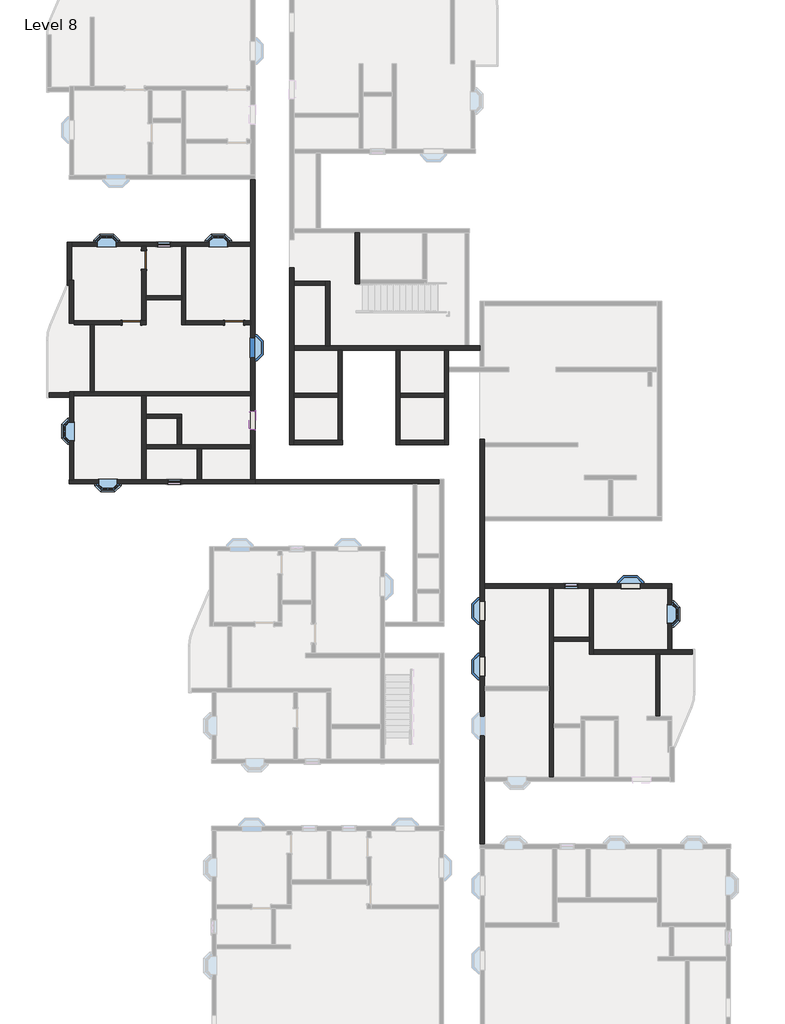
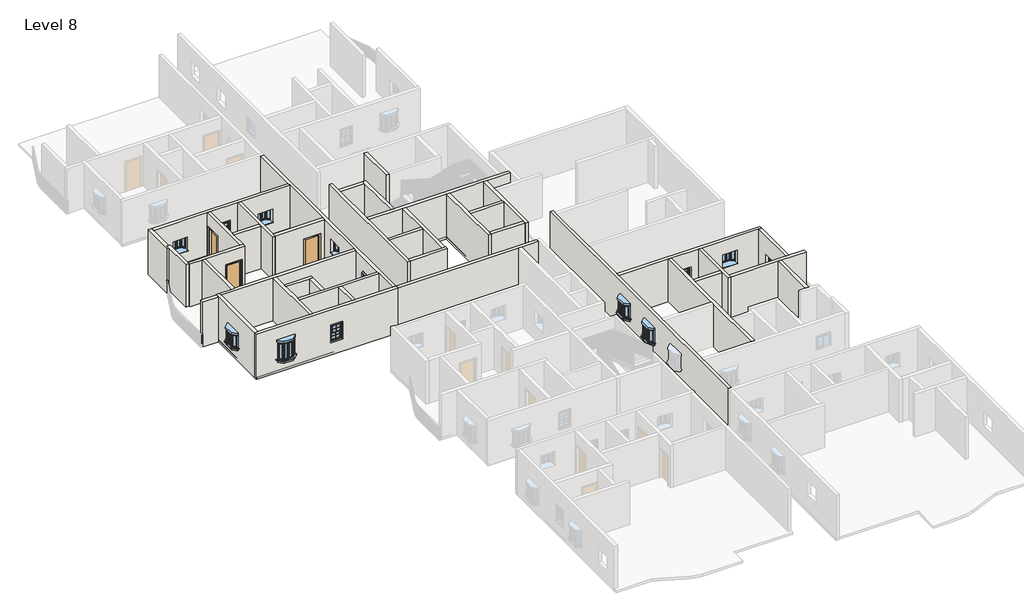
# One storey, part 3 of 14: 40 walls, 13 windows, 3 doors.
# Revit data of these elements (continued)
# Element 25 (IfcWall, "9\"")
#   Top Offset = 0' - 0"
#   Base Offset = 0' - 0"
#   wall height = 10' - 0"
#   Phase Created = New Construction
#   Base Constraint = Level 8
#   Top Constraint = Level 9
#   Materials on its faces: "Default Wall", "Parking Stripe"
# Element 26 (IfcWall, "9\"")
#   Top Offset = 0' - 0"
#   Base Offset = 0' - 0"
#   wall height = 10' - 0"
#   Phase Created = New Construction
#   Base Constraint = Level 8
#   Top Constraint = Level 9
#   Materials on its faces: "Default Wall", "Earth"
# Element 27 (IfcWall, "9\"")
#   Top Offset = 0' - 0"
#   Base Offset = 0' - 0"
#   wall height = 10' - 0"
#   Phase Created = New Construction
#   Base Constraint = Level 8
#   Top Constraint = Level 9
#   Materials on its faces: "Default Wall", "Default Mass Interior Wall"
# Element 28 (IfcWall, "9\"")
#   Top Offset = 0' - 0"
#   Base Offset = 0' - 0"
#   wall height = 10' - 0"
#   Phase Created = New Construction
#   Base Constraint = Level 8
#   Top Constraint = Level 9
#   Materials on its faces: "Default Wall"
# Element 29 (IfcWall, "9\"")
#   Top Offset = 0' - 0"
#   Base Offset = 0' - 0"
#   wall height = 10' - 0"
#   Phase Created = New Construction
#   Base Constraint = Level 8
#   Top Constraint = Level 9
#   Materials on its faces: "Default Wall", "Default Mass Interior Wall", "Earth"
# Elements 30, 33, 34, 35, 36, 37, 38, 39, 40, 41 (IfcWall, "9\" w")
#   Top Offset = 0' - 0"
#   Base Offset = 0' - 0"
#   wall height = 10' - 0"
#   Phase Created = New Construction
#   Base Constraint = Level 8
#   Top Constraint = Level 9
#   Materials on its faces: "Default Wall"
# Element 31 (IfcWall, "9\" w")
#   Top Offset = 0' - 0"
#   Base Offset = 0' - 0"
#   wall height = 10' - 0"
#   Phase Created = New Construction
#   Base Constraint = Level 8
#   Top Constraint = Level 9
#   Materials on its faces: "Default Wall", "Earth"
# Element 32 (IfcWall, "9\" w")
#   Top Offset = 0' - 0"
#   Base Offset = 0' - 0"
#   wall height = 10' - 0"
#   Phase Created = New Construction
#   Base Constraint = Level 8
#   Top Constraint = Level 9
#   Materials on its faces: "Default Wall", "Brick, Soldier Course"
# Element 42 (IfcWall, "9\" w")
#   Top Offset = 0' - 0"
#   Base Offset = 0' - 0"
#   wall height = 10' - 0"
#   Phase Created = New Construction
#   Base Constraint = Level 8
#   Top Constraint = Level 9
#   Materials on its faces: "Default Wall", "Wood - Stained"
# Element 43 (IfcWall, "9\" w")
#   Top Offset = 0' - 0"
#   Base Offset = 0' - 0"
#   wall height = 10' - 0"
#   Phase Created = New Construction
#   Base Constraint = Level 8
#   Top Constraint = Level 9
#   Materials on its faces: "Default Wall", "Acoustic Ceiling Tile 24 x 24"
# Element 44 (IfcWindow, "910x1210mm")
#   Mark = "471"
#   Phase Created = New Construction
#   Materials on its faces: "Window Frame", "Glass"
# Element 45 (IfcWindow, "910x910mm")
#   Mark = "447"
#   Phase Created = New Construction
#   Materials on its faces: "Window Frame", "Glass"
# Element 46 (IfcWindow, "910x910mm")
#   Mark = "448"
#   Phase Created = New Construction
#   Materials on its faces: "Window Frame", "Glass"
# Element 47 (IfcWindow, "910x910mm")
#   Mark = "420"
#   Phase Created = New Construction
#   Materials on its faces: "Window Frame", "Glass"
# Element 48 (IfcWindow, "910x910mm")
#   Mark = "421"
#   Phase Created = New Construction
#   Materials on its faces: "Window Frame", "Glass"
# Element 49 (IfcWindow, "910x910mm")
#   Mark = "422"
#   Phase Created = New Construction
#   Materials on its faces: "Window Frame", "Glass"
# Element 50 (IfcWindow, "910x910mm")
#   Mark = "423"
#   Phase Created = New Construction
#   Materials on its faces: "Window Frame", "Glass"
# Element 51 (IfcWindow, "910x910mm")
#   Mark = "445"
#   Phase Created = New Construction
#   Materials on its faces: "Window Frame", "Glass"
# Element 52 (IfcWindow, "910x910mm")
#   Mark = "446"
#   Phase Created = New Construction
#   Materials on its faces: "Window Frame", "Glass"
# Element 53 (IfcWindow, "Window-Double-Hung : 26\" x 42\"")
#   Mark = "469"
#   Window Inset = 0' - 0"
#   Interior Wall Closure = 0' - 1 1/2"
#   Frame Extension = 0' - 1 1/4"
#   Exterior Wall Closure = 0' - 0 1/2"
#   Interior Trim Visibility = yes
#   Indicator Visibility = yes
#   Exterior Trim Visibility = yes
#   Phase Created = New Construction
#   Materials on its faces: "Wood - Stained", "Glass", "Clad - White"
# Element 54 (IfcWindow, "Window-Double-Hung : 26\" x 42\"")
#   Mark = "458"
#   Window Inset = 0' - 0"
#   Interior Wall Closure = 0' - 1 1/2"
#   Frame Extension = 0' - 1 1/4"
#   Exterior Wall Closure = 0' - 0 1/2"
#   Interior Trim Visibility = yes
#   Indicator Visibility = yes
#   Exterior Trim Visibility = yes
#   Phase Created = New Construction
#   Materials on its faces: "Wood - Stained", "Glass", "Clad - White"
# Element 55 (IfcWindow, "Window-Double-Hung : 26\" x 42\"")
#   Mark = "459"
#   Window Inset = 0' - 0"
#   Interior Wall Closure = 0' - 1 1/2"
#   Frame Extension = 0' - 1 1/4"
#   Exterior Wall Closure = 0' - 0 1/2"
#   Interior Trim Visibility = yes
#   Indicator Visibility = yes
#   Exterior Trim Visibility = yes
#   Phase Created = New Construction
#   Materials on its faces: "Wood - Stained", "Glass", "Clad - White"
# Element 56 (IfcWindow, "Windows_Sgl_w-Glazing_Bars : 910x910mm")
#   Mark = "454"
#   Phase Created = New Construction
#   Materials on its faces: "Window Frame", "Glass"
# Materials
#   "Door - Panel": class "Wood", colour RGB 210 159 95, transparency 0, Cost = 0
#   "Door - Frame": colour RGB 118 70 51, transparency 0, Cost = 0
#   "Window Frame": colour RGB 249 249 249, transparency 0
#   "Glass": class "Glass", colour RGB 0 128 192, transparency 0.75, Description = "Soda Lime Glass", Cost = 0
#   "Wood - Stained": class "Wood", colour RGB 224 178 126, transparency 0, Cost = 0
#   "Clad - White": class "Wood", colour RGB 242 242 238, transparency 0, Cost = 0
#   "Default Wall": colour RGB 128 128 128, transparency 0, Cost = 0
#   "Water": class "Liquid", colour RGB 108 195 217, transparency 0.7, Description = "Water", Cost = 0
#   "Earth": class "Generic", colour RGB 97 75 62, transparency 0, Description = "Soil", Cost = 0
#   "Cherry": class "Wood", colour RGB 226 177 128, transparency 0, Description = "Prunus Serotina", Cost = 0
#   "Parking Stripe": class "Paint", colour RGB 250 250 91, transparency 0, Cost = 0
#   "Default Mass Interior Wall": class "Generic", colour RGB 195 229 126, transparency 0, Cost = 0
#   "Brick, Soldier Course": class "Masonry", colour RGB 170 98 104, transparency 0, Description = "Common brick soldier coursed", Cost = 0
#   "Acoustic Ceiling Tile 24 x 24": class "Generic", colour RGB 232 232 232, transparency 0, Description = "Acoustic Ceiling Tile 24 x 24", Cost = 0
